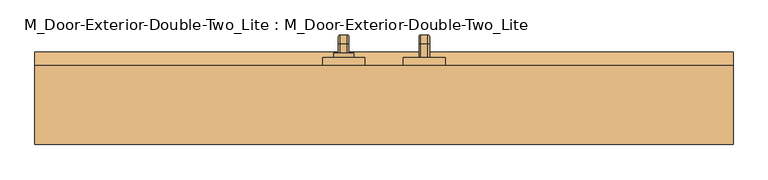
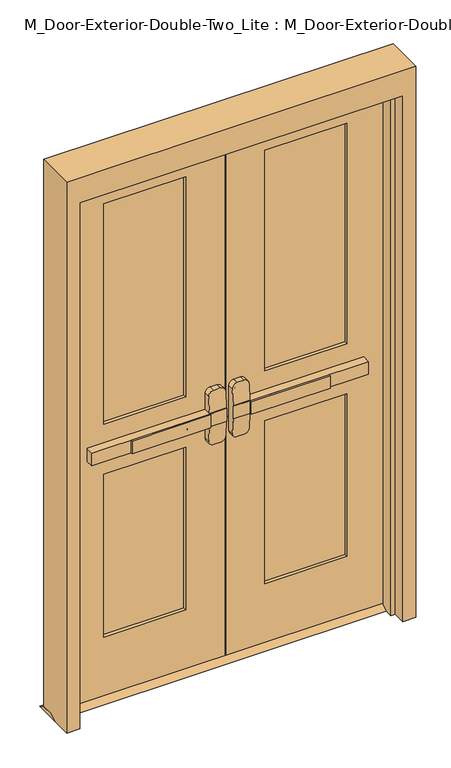
"""IFC4 building model written with IfcOpenShell, lengths in millimetres: door geometry, M_Door-Exterior-Double-Two_Lite : M_Door-Exterior-Double-Two_Lite."""

from ifc_helpers import new_model, si_unit, point, frame, frame_2d, origin, place, context, project, spatial, polyline, circle_curve, ellipse_curve, trimmed, segment, composite_curve, outline, extrude, faceted_brep, source, transform, mapped, element, save
from ifc_brep_helpers import plane_surface, cylinder_surface, revolved_surface, advanced_brep


def m_door_exterior_double_two_lite_m_door_exterior_double_two_f203ad21(model_context):
    return source(origin(), model_context, "Body", "SolidModel", [
        extrude(outline(polyline([(-373.6, 12.55), (-373.6, 18.9), (-76.2, 18.9), (-76.2, 12.55), (-373.6, 12.55)])), frame((0.0, 0.0, 974.6), z_axis=(0.0, 0.0, 1.0), x_axis=(1.0, 0.0, 0.0)), (0.0, 0.0, 1.0), 50.8),
        advanced_brep(
        [(-12.7, 18.9, 1025.4), (-76.2, 18.9, 1025.4), (-522.3, 18.9, 1025.4), (-522.3, 18.9, 974.6), (-76.2, 18.9, 974.6), (-12.7, 18.9, 974.6), (-522.3, 50.65, 1025.4), (-76.2, 50.65, 1025.4), (-76.2, 50.65, 1088.9), (-57.15, 50.65, 1107.95), (-31.75, 50.65, 1107.95), (-12.7, 50.65, 1088.9), (-12.7, 50.65, 911.1), (-31.75, 50.65, 892.05), (-57.15, 50.65, 892.05), (-76.2, 50.65, 911.1), (-76.2, 50.65, 974.6), (-522.3, 50.65, 974.6), (-12.7, 22.0752467, 1025.4), (-76.2, 22.0752467, 1025.4), (-12.7, 22.0752467, 974.6), (-12.7, 27.0854269, 911.1), (-12.7, 27.0854269, 1088.9), (-76.2, 22.0752467, 974.6), (-76.2, 27.0854269, 1088.9), (-76.2, 27.0854269, 911.1), (-57.15, 28.588481, 1107.95), (-31.75, 28.588481, 1107.95), (-31.75, 28.588481, 892.05), (-57.15, 28.588481, 892.05)],
        [
            (0, 1),
            (1, 2),
            (2, 3),
            (3, 4),
            (4, 5),
            (5, 0),
            (6, 7),
            (7, 8),
            (8, 9, circle_curve(frame((-57.15, 50.65, 1088.9), z_axis=(0.0, 1.0, 0.0), x_axis=(-1.0, 0.0, 0.0)), 19.05)),
            (9, 10),
            (10, 11, circle_curve(frame((-31.75, 50.65, 1088.9), z_axis=(0.0, 1.0, 0.0), x_axis=(-1.0, 0.0, 0.0)), 19.05)),
            (11, 12),
            (12, 13, circle_curve(frame((-31.75, 50.65, 911.1), z_axis=(0.0, 1.0, 0.0), x_axis=(-1.0, 0.0, 0.0)), 19.05)),
            (13, 14),
            (14, 15, circle_curve(frame((-57.15, 50.65, 911.1), z_axis=(0.0, 1.0, 0.0), x_axis=(-1.0, 0.0, 0.0)), 19.05)),
            (15, 16),
            (16, 17),
            (17, 6),
            (0, 18),
            (18, 19),
            (19, 7),
            (6, 2),
            (5, 20),
            (20, 21),
            (21, 12),
            (11, 22),
            (22, 18),
            (16, 23),
            (23, 20),
            (3, 17),
            (19, 24),
            (24, 8),
            (15, 25),
            (25, 23),
            (9, 26),
            (26, 27),
            (27, 10),
            (13, 28),
            (28, 29),
            (29, 14),
            (29, 25, ellipse_curve(frame((-57.15, 27.0854269, 911.1), z_axis=(0.0, 0.9969018152893365, 0.07865602756830282), x_axis=(0.0, -0.07865602756830208, 0.9969018152893365)), 19.1092038, 19.05)),
            (24, 26, ellipse_curve(frame((-57.15, 27.0854269, 1088.9), z_axis=(0.0, 0.9969018152893376, -0.07865602756828934), x_axis=(0.0, -0.078656027568288, -0.9969018152893377)), 19.1092038, 19.05)),
            (27, 22, ellipse_curve(frame((-31.75, 27.0854269, 1088.9), z_axis=(0.0, 0.9969018152893376, -0.07865602756828934), x_axis=(0.0, -0.078656027568288, -0.9969018152893377)), 19.1092038, 19.05)),
            (21, 28, ellipse_curve(frame((-31.75, 27.0854269, 911.1), z_axis=(0.0, 0.9969018152893365, 0.07865602756830282), x_axis=(0.0, -0.07865602756830208, 0.9969018152893365)), 19.1092038, 19.05)),
        ],
        [
            plane_surface(frame((-12.7, 18.9, 1025.4), z_axis=(0.0, -1.0, 0.0), x_axis=(1.0, 0.0, 0.0))),
            plane_surface(frame((-12.7, 50.65, 1025.4), z_axis=(0.0, 1.0, 0.0), x_axis=(-1.0, 0.0, 0.0))),
            plane_surface(frame((-522.3, 18.9, 1025.4), z_axis=(0.0, 0.0, 1.0), x_axis=(0.0, 1.0, 0.0))),
            plane_surface(frame((-12.7, 18.9, 1025.4), z_axis=(1.0, 0.0, 0.0), x_axis=(0.0, 1.0, 0.0))),
            plane_surface(frame((-12.7, 18.9, 974.6), z_axis=(0.0, 0.0, -1.0), x_axis=(0.0, 1.0, 0.0))),
            plane_surface(frame((-522.3, 18.9, 974.6), z_axis=(-1.0, 0.0, 0.0), x_axis=(0.0, 1.0, 0.0))),
            plane_surface(frame((-76.2, 22.0752467, 911.1), z_axis=(-1.0, 0.0, 0.0), x_axis=(0.0, 1.0, 0.0))),
            plane_surface(frame((-57.15, 22.0752467, 1107.95), z_axis=(0.0, 0.0, 1.0), x_axis=(0.0, 1.0, 0.0))),
            plane_surface(frame((-31.75, 22.0752467, 892.05), z_axis=(0.0, 0.0, -1.0), x_axis=(0.0, 1.0, 0.0))),
            cylinder_surface(frame((-57.15, 50.65, 911.1), z_axis=(0.0, -1.0, 0.0), x_axis=(-1.0, 0.0, 0.0)), 19.05),
            cylinder_surface(frame((-57.15, 50.65, 1088.9), z_axis=(0.0, -1.0, 0.0), x_axis=(-1.0, 0.0, 0.0)), 19.05),
            cylinder_surface(frame((-31.75, 50.65, 1088.9), z_axis=(0.0, -1.0, 0.0), x_axis=(-1.0, 0.0, 0.0)), 19.05),
            cylinder_surface(frame((-31.75, 50.65, 911.1), z_axis=(0.0, -1.0, 0.0), x_axis=(-1.0, 0.0, 0.0)), 19.05),
            plane_surface(frame((-76.2, 22.0752467, 1025.4), z_axis=(0.0, -0.9969018152893376, 0.07865602756828934), x_axis=(1.0, 0.0, 0.0))),
            plane_surface(frame((-76.2, 28.588481, 892.05), z_axis=(0.0, -0.9969018152893365, -0.07865602756830282), x_axis=(1.0, 0.0, 0.0))),
        ],
        [
            (0, [[1, 2, 3, 4, 5, 6]]),
            (1, [[7, 8, 9, 10, 11, 12, 13, 14, 15, 16, 17, 18]]),
            (2, [[-2, -1, 19, 20, 21, -7, 22]]),
            (3, [[23, 24, 25, -12, 26, 27, -19, -6]]),
            (4, [[-17, 28, 29, -23, -5, -4, 30]]),
            (5, [[-22, -18, -30, -3]]),
            (6, [[-21, 31, 32, -8]]),
            (6, [[33, 34, -28, -16]]),
            (7, [[35, 36, 37, -10]]),
            (8, [[38, 39, 40, -14]]),
            (9, [[-40, 41, -33, -15]]),
            (10, [[-32, 42, -35, -9]]),
            (11, [[-37, 43, -26, -11]]),
            (12, [[-25, 44, -38, -13]]),
            (13, [[-27, -43, -36, -42, -31, -20]]),
            (14, [[-29, -34, -41, -39, -44, -24]]),
        ],
    ),
        extrude(outline(polyline([(95.65, 15.0), (121.05, 0.0), (25.25, 0.0), (50.65, 15.0), (95.65, 15.0)])), frame((-659.6, 0.0, 0.0), z_axis=(1.0, 0.0, 0.0), x_axis=(0.0, 1.0, 0.0)), (0.0, 0.0, 1.0), 1319.2),
        extrude(outline(polyline([(373.6, 12.55), (76.2, 12.55), (76.2, 18.9), (373.6, 18.9), (373.6, 12.55)])), frame((0.0, 0.0, 974.6), z_axis=(0.0, 0.0, 1.0), x_axis=(1.0, 0.0, 0.0)), (0.0, 0.0, 1.0), 50.8),
        advanced_brep(
        [(12.7, 18.9, 1025.4), (12.7, 18.9, 974.6), (76.2, 18.9, 974.6), (522.3, 18.9, 974.6), (522.3, 18.9, 1025.4), (76.2, 18.9, 1025.4), (522.3, 50.65, 1025.4), (522.3, 50.65, 974.6), (76.2, 50.65, 974.6), (76.2, 50.65, 911.1), (57.15, 50.65, 892.05), (31.75, 50.65, 892.05), (12.7, 50.65, 911.1), (12.7, 50.65, 1088.9), (31.75, 50.65, 1107.95), (57.15, 50.65, 1107.95), (76.2, 50.65, 1088.9), (76.2, 50.65, 1025.4), (76.2, 22.0752467, 1025.4), (12.7, 22.0752467, 1025.4), (12.7, 27.0854269, 1088.9), (12.7, 27.0854269, 911.1), (12.7, 22.0752467, 974.6), (76.2, 22.0752467, 974.6), (76.2, 27.0854269, 911.1), (76.2, 27.0854269, 1088.9), (31.75, 28.588481, 1107.95), (57.15, 28.588481, 1107.95), (57.15, 28.588481, 892.05), (31.75, 28.588481, 892.05)],
        [
            (0, 1),
            (1, 2),
            (2, 3),
            (3, 4),
            (4, 5),
            (5, 0),
            (6, 7),
            (7, 8),
            (8, 9),
            (9, 10, circle_curve(frame((57.15, 50.65, 911.1), z_axis=(0.0, 1.0, 0.0), x_axis=(1.0, 0.0, 0.0)), 19.05)),
            (10, 11),
            (11, 12, circle_curve(frame((31.75, 50.65, 911.1), z_axis=(0.0, 1.0, 0.0), x_axis=(1.0, 0.0, 0.0)), 19.05)),
            (12, 13),
            (13, 14, circle_curve(frame((31.75, 50.65, 1088.9), z_axis=(0.0, 1.0, 0.0), x_axis=(1.0, 0.0, 0.0)), 19.05)),
            (14, 15),
            (15, 16, circle_curve(frame((57.15, 50.65, 1088.9), z_axis=(0.0, 1.0, 0.0), x_axis=(1.0, 0.0, 0.0)), 19.05)),
            (16, 17),
            (17, 6),
            (4, 6),
            (17, 18),
            (18, 19),
            (19, 0),
            (19, 20),
            (20, 13),
            (12, 21),
            (21, 22),
            (22, 1),
            (7, 3),
            (22, 23),
            (23, 8),
            (23, 24),
            (24, 9),
            (16, 25),
            (25, 18),
            (14, 26),
            (26, 27),
            (27, 15),
            (10, 28),
            (28, 29),
            (29, 11),
            (24, 28, ellipse_curve(frame((57.15, 27.0854269, 911.1), z_axis=(0.0, 0.9969018152893365, 0.07865602756830282), x_axis=(0.0, -0.07865602756830208, 0.9969018152893365)), 19.1092038, 19.05)),
            (27, 25, ellipse_curve(frame((57.15, 27.0854269, 1088.9), z_axis=(0.0, 0.9969018152893376, -0.07865602756828934), x_axis=(0.0, -0.078656027568288, -0.9969018152893377)), 19.1092038, 19.05)),
            (20, 26, ellipse_curve(frame((31.75, 27.0854269, 1088.9), z_axis=(0.0, 0.9969018152893376, -0.07865602756828934), x_axis=(0.0, -0.078656027568288, -0.9969018152893377)), 19.1092038, 19.05)),
            (29, 21, ellipse_curve(frame((31.75, 27.0854269, 911.1), z_axis=(0.0, 0.9969018152893365, 0.07865602756830282), x_axis=(0.0, -0.07865602756830208, 0.9969018152893365)), 19.1092038, 19.05)),
        ],
        [
            plane_surface(frame((12.7, 18.9, 1025.4), z_axis=(0.0, -1.0, 0.0), x_axis=(-1.0, 0.0, 0.0))),
            plane_surface(frame((12.7, 50.65, 1025.4), z_axis=(0.0, 1.0, 0.0), x_axis=(1.0, 0.0, 0.0))),
            plane_surface(frame((522.3, 18.9, 1025.4), z_axis=(0.0, 0.0, 1.0), x_axis=(0.0, 1.0, 0.0))),
            plane_surface(frame((12.7, 18.9, 1025.4), z_axis=(-1.0, 0.0, 0.0), x_axis=(0.0, 1.0, 0.0))),
            plane_surface(frame((12.7, 18.9, 974.6), z_axis=(0.0, 0.0, -1.0), x_axis=(0.0, 1.0, 0.0))),
            plane_surface(frame((522.3, 18.9, 974.6), z_axis=(1.0, 0.0, 0.0), x_axis=(0.0, 1.0, 0.0))),
            plane_surface(frame((76.2, 22.0752467, 911.1), z_axis=(1.0, 0.0, 0.0), x_axis=(0.0, 1.0, 0.0))),
            plane_surface(frame((57.15, 22.0752467, 1107.95), z_axis=(0.0, 0.0, 1.0), x_axis=(0.0, 1.0, 0.0))),
            plane_surface(frame((31.75, 22.0752467, 892.05), z_axis=(0.0, 0.0, -1.0), x_axis=(0.0, 1.0, 0.0))),
            cylinder_surface(frame((57.15, 50.65, 911.1), z_axis=(0.0, -1.0, 0.0), x_axis=(1.0, 0.0, 0.0)), 19.05),
            cylinder_surface(frame((57.15, 50.65, 1088.9), z_axis=(0.0, -1.0, 0.0), x_axis=(1.0, 0.0, 0.0)), 19.05),
            cylinder_surface(frame((31.75, 50.65, 1088.9), z_axis=(0.0, -1.0, 0.0), x_axis=(1.0, 0.0, 0.0)), 19.05),
            cylinder_surface(frame((31.75, 50.65, 911.1), z_axis=(0.0, -1.0, 0.0), x_axis=(1.0, 0.0, 0.0)), 19.05),
            plane_surface(frame((76.2, 22.0752467, 1025.4), z_axis=(0.0, -0.9969018152893376, 0.07865602756828934), x_axis=(-1.0, 0.0, 0.0))),
            plane_surface(frame((76.2, 28.588481, 892.05), z_axis=(0.0, -0.9969018152893365, -0.07865602756830282), x_axis=(-1.0, 0.0, 0.0))),
        ],
        [
            (0, [[1, 2, 3, 4, 5, 6]]),
            (1, [[7, 8, 9, 10, 11, 12, 13, 14, 15, 16, 17, 18]]),
            (2, [[19, -18, 20, 21, 22, -6, -5]]),
            (3, [[-1, -22, 23, 24, -13, 25, 26, 27]]),
            (4, [[28, -3, -2, -27, 29, 30, -8]]),
            (5, [[-4, -28, -7, -19]]),
            (6, [[-9, -30, 31, 32]]),
            (6, [[-17, 33, 34, -20]]),
            (7, [[-15, 35, 36, 37]]),
            (8, [[-11, 38, 39, 40]]),
            (9, [[-10, -32, 41, -38]]),
            (10, [[-16, -37, 42, -33]]),
            (11, [[-14, -24, 43, -35]]),
            (12, [[-12, -40, 44, -25]]),
            (13, [[-21, -34, -42, -36, -43, -23]]),
            (14, [[-26, -44, -39, -41, -31, -29]]),
        ],
    ),
        advanced_brep(
        [(66.2, 110.65, 1001.190625), (66.2, 110.65, 998.809375), (69.771875, 110.65, 995.2375), (82.6284594, 110.65, 995.2375), (86.2, 110.65, 998.8090406), (86.2, 110.65, 1001.190625), (82.628125, 110.65, 1004.7625), (69.771875, 110.65, 1004.7625), (66.2, 110.65, 874.609375), (69.771875, 110.65, 871.0375), (82.628125, 110.65, 871.0375), (86.2, 110.65, 874.609375), (86.2, 110.65, 876.9909594), (82.6284594, 110.65, 880.5625), (69.771875, 110.65, 880.5625), (66.2, 110.65, 876.990625), (66.2, 136.05, 1001.190625), (66.2, 149.940625, 987.3), (66.2, 149.940625, 888.5), (66.2, 136.05, 874.609375), (66.2, 136.05, 876.990625), (66.2, 147.559375, 888.5), (66.2, 147.559375, 987.3), (66.2, 136.05, 998.809375), (69.771875, 136.05, 995.2375), (82.6284594, 136.05, 995.2375), (86.2, 136.05, 998.8090406), (86.2, 147.5590406, 987.3), (86.2, 147.5590406, 888.5), (86.2, 136.05, 876.9909594), (86.2, 136.05, 874.609375), (86.2, 149.940625, 888.5), (86.2, 149.940625, 987.3), (86.2, 136.05, 1001.190625), (82.628125, 136.05, 1004.7625), (69.771875, 136.05, 1004.7625), (69.771875, 143.9875, 987.3), (82.6284594, 143.9875, 987.3), (82.628125, 153.5125, 987.3), (69.771875, 153.5125, 987.3), (69.771875, 143.9875, 888.5), (82.6284594, 143.9875, 888.5), (82.628125, 153.5125, 888.5), (69.771875, 153.5125, 888.5), (69.771875, 136.05, 880.5625), (82.6284594, 136.05, 880.5625), (82.628125, 136.05, 871.0375), (69.771875, 136.05, 871.0375)],
        [
            (0, 1),
            (1, 2, circle_curve(frame((69.771875, 110.65, 998.809375), z_axis=(0.0, -1.0, 0.0), x_axis=(0.0, 0.0, 1.0)), 3.571875)),
            (2, 3),
            (3, 4, circle_curve(frame((82.6284594, 110.65, 998.8090406), z_axis=(0.0, -1.0, 0.0), x_axis=(0.0, 0.0, 1.0)), 3.5715406)),
            (4, 5),
            (5, 6, circle_curve(frame((82.628125, 110.65, 1001.190625), z_axis=(0.0, -1.0, 0.0), x_axis=(0.0, 0.0, 1.0)), 3.571875)),
            (6, 7),
            (7, 0, circle_curve(frame((69.771875, 110.65, 1001.190625), z_axis=(0.0, -1.0, 0.0), x_axis=(0.0, 0.0, 1.0)), 3.571875)),
            (8, 9, circle_curve(frame((69.771875, 110.65, 874.609375), z_axis=(0.0, -1.0, 0.0), x_axis=(0.0, 0.0, -1.0)), 3.571875)),
            (9, 10),
            (10, 11, circle_curve(frame((82.628125, 110.65, 874.609375), z_axis=(0.0, -1.0, 0.0), x_axis=(0.0, 0.0, -1.0)), 3.571875)),
            (11, 12),
            (12, 13, circle_curve(frame((82.6284594, 110.65, 876.9909594), z_axis=(0.0, -1.0, 0.0), x_axis=(0.0, 0.0, -1.0)), 3.5715406)),
            (13, 14),
            (14, 15, circle_curve(frame((69.771875, 110.65, 876.990625), z_axis=(0.0, -1.0, 0.0), x_axis=(0.0, 0.0, -1.0)), 3.571875)),
            (15, 8),
            (0, 16),
            (16, 17, circle_curve(frame((66.2, 136.05, 987.3), z_axis=(-1.0, 0.0, 0.0), x_axis=(0.0, 0.0, 1.0)), 13.890625)),
            (17, 18),
            (18, 19, circle_curve(frame((66.2, 136.05, 888.5), z_axis=(-1.0, 0.0, 0.0), x_axis=(0.0, 1.0, 0.0)), 13.890625)),
            (19, 8),
            (15, 20),
            (20, 21, circle_curve(frame((66.2, 136.05, 888.5), z_axis=(1.0, 0.0, 0.0), x_axis=(0.0, 1.0, 0.0)), 11.509375)),
            (21, 22),
            (22, 23, circle_curve(frame((66.2, 136.05, 987.3), z_axis=(1.0, 0.0, 0.0), x_axis=(0.0, 0.0, 1.0)), 11.509375)),
            (23, 1),
            (23, 24, circle_curve(frame((69.771875, 136.05, 998.809375), z_axis=(0.0, -1.0, 0.0), x_axis=(0.0, 0.0, 1.0)), 3.571875)),
            (24, 2),
            (24, 25),
            (25, 3),
            (25, 26, circle_curve(frame((82.6284594, 136.05, 998.8090406), z_axis=(0.0, -1.0, 0.0), x_axis=(0.0, 0.0, 1.0)), 3.5715406)),
            (26, 4),
            (26, 27, circle_curve(frame((86.2, 136.05, 987.3), z_axis=(-1.0, 0.0, 0.0), x_axis=(0.0, 0.0, 1.0)), 11.5090406)),
            (27, 28),
            (28, 29, circle_curve(frame((86.2, 136.05, 888.5), z_axis=(-1.0, 0.0, 0.0), x_axis=(0.0, 1.0, 0.0)), 11.5090406)),
            (29, 12),
            (11, 30),
            (30, 31, circle_curve(frame((86.2, 136.05, 888.5), z_axis=(1.0, 0.0, 0.0), x_axis=(0.0, 1.0, 0.0)), 13.890625)),
            (31, 32),
            (32, 33, circle_curve(frame((86.2, 136.05, 987.3), z_axis=(1.0, 0.0, 0.0), x_axis=(0.0, 0.0, 1.0)), 13.890625)),
            (33, 5),
            (33, 34, circle_curve(frame((82.628125, 136.05, 1001.190625), z_axis=(0.0, -1.0, 0.0), x_axis=(0.0, 0.0, 1.0)), 3.571875)),
            (34, 6),
            (34, 35),
            (35, 7),
            (35, 16, circle_curve(frame((69.771875, 136.05, 1001.190625), z_axis=(0.0, -1.0, 0.0), x_axis=(0.0, 0.0, 1.0)), 3.571875)),
            (36, 24, circle_curve(frame((69.771875, 136.05, 987.3), z_axis=(1.0, 0.0, 0.0), x_axis=(0.0, 0.0, 1.0)), 7.9375)),
            (22, 36, circle_curve(frame((69.771875, 147.559375, 987.3), z_axis=(0.0, 0.0, 1.0), x_axis=(0.0, 1.0, 0.0)), 3.571875)),
            (37, 25, circle_curve(frame((82.6284594, 136.05, 987.3), z_axis=(1.0, 0.0, 0.0), x_axis=(0.0, 0.0, 1.0)), 7.9375)),
            (36, 37),
            (37, 27, circle_curve(frame((82.6284594, 147.5590406, 987.3), z_axis=(0.0, 0.0, 1.0), x_axis=(0.0, 1.0, 0.0)), 3.5715406)),
            (38, 34, circle_curve(frame((82.628125, 136.05, 987.3), z_axis=(1.0, 0.0, 0.0), x_axis=(0.0, 0.0, 1.0)), 17.4625)),
            (32, 38, circle_curve(frame((82.628125, 149.940625, 987.3), z_axis=(0.0, 0.0, 1.0), x_axis=(0.0, 1.0, 0.0)), 3.571875)),
            (39, 35, circle_curve(frame((69.771875, 136.05, 987.3), z_axis=(1.0, 0.0, 0.0), x_axis=(0.0, 0.0, 1.0)), 17.4625)),
            (38, 39),
            (39, 17, circle_curve(frame((69.771875, 149.940625, 987.3), z_axis=(0.0, 0.0, 1.0), x_axis=(0.0, 1.0, 0.0)), 3.571875)),
            (21, 40, circle_curve(frame((69.771875, 147.559375, 888.5), z_axis=(0.0, 0.0, 1.0), x_axis=(0.0, 1.0, 0.0)), 3.571875)),
            (40, 36),
            (40, 41),
            (41, 37),
            (41, 28, circle_curve(frame((82.6284594, 147.5590406, 888.5), z_axis=(0.0, 0.0, 1.0), x_axis=(0.0, 1.0, 0.0)), 3.5715406)),
            (31, 42, circle_curve(frame((82.628125, 149.940625, 888.5), z_axis=(0.0, 0.0, 1.0), x_axis=(0.0, 1.0, 0.0)), 3.571875)),
            (42, 38),
            (42, 43),
            (43, 39),
            (43, 18, circle_curve(frame((69.771875, 149.940625, 888.5), z_axis=(0.0, 0.0, 1.0), x_axis=(0.0, 1.0, 0.0)), 3.571875)),
            (44, 40, circle_curve(frame((69.771875, 136.05, 888.5), z_axis=(1.0, 0.0, 0.0), x_axis=(0.0, 1.0, 0.0)), 7.9375)),
            (20, 44, circle_curve(frame((69.771875, 136.05, 876.990625), z_axis=(0.0, 1.0, 0.0), x_axis=(0.0, 0.0, -1.0)), 3.571875)),
            (45, 41, circle_curve(frame((82.6284594, 136.05, 888.5), z_axis=(1.0, 0.0, 0.0), x_axis=(0.0, 1.0, 0.0)), 7.9375)),
            (44, 45),
            (45, 29, circle_curve(frame((82.6284594, 136.05, 876.9909594), z_axis=(0.0, 1.0, 0.0), x_axis=(0.0, 0.0, -1.0)), 3.5715406)),
            (46, 42, circle_curve(frame((82.628125, 136.05, 888.5), z_axis=(1.0, 0.0, 0.0), x_axis=(0.0, 1.0, 0.0)), 17.4625)),
            (30, 46, circle_curve(frame((82.628125, 136.05, 874.609375), z_axis=(0.0, 1.0, 0.0), x_axis=(0.0, 0.0, -1.0)), 3.571875)),
            (47, 43, circle_curve(frame((69.771875, 136.05, 888.5), z_axis=(1.0, 0.0, 0.0), x_axis=(0.0, 1.0, 0.0)), 17.4625)),
            (46, 47),
            (47, 19, circle_curve(frame((69.771875, 136.05, 874.609375), z_axis=(0.0, 1.0, 0.0), x_axis=(0.0, 0.0, -1.0)), 3.571875)),
            (14, 44),
            (13, 45),
            (10, 46),
            (9, 47),
        ],
        [
            plane_surface(frame((76.2, 110.65, 1000.0), z_axis=(0.0, -1.0, 0.0), x_axis=(1.0, 0.0, 0.0))),
            plane_surface(frame((76.2, 110.65, 875.8), z_axis=(0.0, -1.0, 0.0), x_axis=(1.0, 0.0, 0.0))),
            plane_surface(frame((66.2, 110.65, 1001.190625), z_axis=(-1.0, 0.0, 0.0), x_axis=(0.0, 1.0, 0.0))),
            cylinder_surface(frame((69.771875, 110.65, 998.809375), z_axis=(0.0, -1.0, 0.0), x_axis=(0.0, 0.0, 1.0)), 3.571875),
            plane_surface(frame((69.771875, 110.65, 995.2375), z_axis=(0.0, 0.0, -1.0), x_axis=(0.0, 1.0, 0.0))),
            cylinder_surface(frame((82.6284594, 110.65, 998.8090406), z_axis=(0.0, -1.0, 0.0), x_axis=(0.0, 0.0, 1.0)), 3.5715406),
            plane_surface(frame((86.2, 110.65, 998.8090406), z_axis=(1.0, 0.0, 0.0), x_axis=(0.0, 1.0, 0.0))),
            cylinder_surface(frame((82.628125, 110.65, 1001.190625), z_axis=(0.0, -1.0, 0.0), x_axis=(0.0, 0.0, 1.0)), 3.571875),
            plane_surface(frame((82.628125, 110.65, 1004.7625), z_axis=(0.0, 0.0, 1.0), x_axis=(0.0, 1.0, 0.0))),
            cylinder_surface(frame((69.771875, 110.65, 1001.190625), z_axis=(0.0, -1.0, 0.0), x_axis=(0.0, 0.0, 1.0)), 3.571875),
            revolved_surface(trimmed(ellipse_curve(frame((69.771875, 136.05, 998.809375), z_axis=(0.0, -1.0, 0.0), x_axis=(0.0, 0.0, 1.0)), 3.571875, 3.571875), [point((66.2, 136.05, 998.809375))], [point((69.771875, 136.05, 995.2375))], True, "CARTESIAN"), (76.2, 136.05, 987.3), (-1.0, 0.0, 0.0)),
            revolved_surface(polyline([(69.771875, 136.05, 995.2375), (82.6284594, 136.05, 995.2375)]), (76.2, 136.05, 987.3), (-1.0, 0.0, 0.0)),
            revolved_surface(trimmed(ellipse_curve(frame((82.6284594, 136.05, 998.8090406), z_axis=(0.0, -1.0, 0.0), x_axis=(0.0, 0.0, 1.0)), 3.5715406, 3.5715406), [point((82.6284594, 136.05, 995.2375))], [point((86.2, 136.05, 998.8090406))], True, "CARTESIAN"), (76.2, 136.05, 987.3), (-1.0, 0.0, 0.0)),
            revolved_surface(trimmed(ellipse_curve(frame((82.628125, 136.05, 1001.190625), z_axis=(0.0, -1.0, 0.0), x_axis=(0.0, 0.0, 1.0)), 3.571875, 3.571875), [point((86.2, 136.05, 1001.190625))], [point((82.628125, 136.05, 1004.7625))], True, "CARTESIAN"), (76.2, 136.05, 987.3), (-1.0, 0.0, 0.0)),
            cylinder_surface(frame((76.2, 136.05, 987.3), z_axis=(-1.0, 0.0, 0.0), x_axis=(0.0, 0.0, 1.0)), 17.4625),
            revolved_surface(trimmed(ellipse_curve(frame((69.771875, 136.05, 1001.190625), z_axis=(0.0, -1.0, 0.0), x_axis=(0.0, 0.0, 1.0)), 3.571875, 3.571875), [point((69.771875, 136.05, 1004.7625))], [point((66.2, 136.05, 1001.190625))], True, "CARTESIAN"), (76.2, 136.05, 987.3), (-1.0, 0.0, 0.0)),
            cylinder_surface(frame((69.771875, 147.559375, 987.3), z_axis=(0.0, 0.0, 1.0), x_axis=(0.0, 1.0, 0.0)), 3.571875),
            plane_surface(frame((69.771875, 143.9875, 987.3), z_axis=(0.0, -1.0, 0.0), x_axis=(0.0, 0.0, -1.0))),
            cylinder_surface(frame((82.6284594, 147.5590406, 987.3), z_axis=(0.0, 0.0, 1.0), x_axis=(0.0, 1.0, 0.0)), 3.5715406),
            cylinder_surface(frame((82.628125, 149.940625, 987.3), z_axis=(0.0, 0.0, 1.0), x_axis=(0.0, 1.0, 0.0)), 3.571875),
            plane_surface(frame((82.628125, 153.5125, 987.3), z_axis=(0.0, 1.0, 0.0), x_axis=(0.0, 0.0, -1.0))),
            cylinder_surface(frame((69.771875, 149.940625, 987.3), z_axis=(0.0, 0.0, 1.0), x_axis=(0.0, 1.0, 0.0)), 3.571875),
            revolved_surface(trimmed(ellipse_curve(frame((69.771875, 147.559375, 888.5), z_axis=(0.0, 0.0, 1.0), x_axis=(0.0, 1.0, 0.0)), 3.571875, 3.571875), [point((66.2, 147.559375, 888.5))], [point((69.771875, 143.9875, 888.5))], True, "CARTESIAN"), (76.2, 136.05, 888.5), (-1.0, 0.0, 0.0)),
            revolved_surface(polyline([(69.771875, 143.9875, 888.5), (82.6284594, 143.9875, 888.5)]), (76.2, 136.05, 888.5), (-1.0, 0.0, 0.0)),
            revolved_surface(trimmed(ellipse_curve(frame((82.6284594, 147.5590406, 888.5), z_axis=(0.0, 0.0, 1.0), x_axis=(0.0, 1.0, 0.0)), 3.5715406, 3.5715406), [point((82.6284594, 143.9875, 888.5))], [point((86.2, 147.5590406, 888.5))], True, "CARTESIAN"), (76.2, 136.05, 888.5), (-1.0, 0.0, 0.0)),
            revolved_surface(trimmed(ellipse_curve(frame((82.628125, 149.940625, 888.5), z_axis=(0.0, 0.0, 1.0), x_axis=(0.0, 1.0, 0.0)), 3.571875, 3.571875), [point((86.2, 149.940625, 888.5))], [point((82.628125, 153.5125, 888.5))], True, "CARTESIAN"), (76.2, 136.05, 888.5), (-1.0, 0.0, 0.0)),
            cylinder_surface(frame((76.2, 136.05, 888.5), z_axis=(-1.0, 0.0, 0.0), x_axis=(0.0, 1.0, 0.0)), 17.4625),
            revolved_surface(trimmed(ellipse_curve(frame((69.771875, 149.940625, 888.5), z_axis=(0.0, 0.0, 1.0), x_axis=(0.0, 1.0, 0.0)), 3.571875, 3.571875), [point((69.771875, 153.5125, 888.5))], [point((66.2, 149.940625, 888.5))], True, "CARTESIAN"), (76.2, 136.05, 888.5), (-1.0, 0.0, 0.0)),
            cylinder_surface(frame((69.771875, 136.05, 876.990625), z_axis=(0.0, 1.0, 0.0), x_axis=(0.0, 0.0, -1.0)), 3.571875),
            plane_surface(frame((69.771875, 136.05, 880.5625), z_axis=(0.0, 0.0, 1.0), x_axis=(0.0, -1.0, 0.0))),
            cylinder_surface(frame((82.6284594, 136.05, 876.9909594), z_axis=(0.0, 1.0, 0.0), x_axis=(0.0, 0.0, -1.0)), 3.5715406),
            cylinder_surface(frame((82.628125, 136.05, 874.609375), z_axis=(0.0, 1.0, 0.0), x_axis=(0.0, 0.0, -1.0)), 3.571875),
            plane_surface(frame((82.628125, 136.05, 871.0375), z_axis=(0.0, 0.0, -1.0), x_axis=(0.0, -1.0, 0.0))),
            cylinder_surface(frame((69.771875, 136.05, 874.609375), z_axis=(0.0, 1.0, 0.0), x_axis=(0.0, 0.0, -1.0)), 3.571875),
        ],
        [
            (0, [[1, 2, 3, 4, 5, 6, 7, 8]]),
            (1, [[9, 10, 11, 12, 13, 14, 15, 16]]),
            (2, [[-1, 17, 18, 19, 20, 21, -16, 22, 23, 24, 25, 26]]),
            (3, [[-2, -26, 27, 28]]),
            (4, [[-3, -28, 29, 30]]),
            (5, [[-4, -30, 31, 32]]),
            (6, [[-5, -32, 33, 34, 35, 36, -12, 37, 38, 39, 40, 41]]),
            (7, [[-6, -41, 42, 43]]),
            (8, [[-7, -43, 44, 45]]),
            (9, [[-8, -45, 46, -17]]),
            (10, [[47, -27, -25, 48]]),
            (11, [[49, -29, -47, 50]]),
            (12, [[-33, -31, -49, 51]]),
            (13, [[52, -42, -40, 53]]),
            (14, [[54, -44, -52, 55]]),
            (15, [[-18, -46, -54, 56]]),
            (16, [[-48, -24, 57, 58]]),
            (17, [[-50, -58, 59, 60]]),
            (18, [[-51, -60, 61, -34]]),
            (19, [[-53, -39, 62, 63]]),
            (20, [[-55, -63, 64, 65]]),
            (21, [[-56, -65, 66, -19]]),
            (22, [[67, -57, -23, 68]]),
            (23, [[69, -59, -67, 70]]),
            (24, [[-35, -61, -69, 71]]),
            (25, [[72, -62, -38, 73]]),
            (26, [[74, -64, -72, 75]]),
            (27, [[-20, -66, -74, 76]]),
            (28, [[-68, -22, -15, 77]]),
            (29, [[-70, -77, -14, 78]]),
            (30, [[-71, -78, -13, -36]]),
            (31, [[-73, -37, -11, 79]]),
            (32, [[-75, -79, -10, 80]]),
            (33, [[-76, -80, -9, -21]]),
        ],
    ),
        extrude(outline(composite_curve([segment(trimmed(circle_curve(frame_2d((1094.2338574, 76.2)), 90.1286291), [point((1175.0, 116.2))], [point((1175.0, 36.2))], False, "CARTESIAN"), True, "CONTINUOUS"), segment(polyline([(1175.0, 36.2), (825.0, 36.2)]), True, "CONTINUOUS"), segment(trimmed(circle_curve(frame_2d((905.7661426, 76.2)), 90.1286291), [point((825.0, 36.2))], [point((825.0, 116.2))], False, "CARTESIAN"), True, "CONTINUOUS"), segment(polyline([(825.0, 116.2), (1175.0, 116.2)]), True, "CONTINUOUS")], self_intersect=False)), frame((0.0, 95.65, 0.0), z_axis=(0.0, 1.0, 0.0), x_axis=(0.0, 0.0, 1.0)), (0.0, 0.0, 1.0), 15.0),
        advanced_brep(
        [(-86.2, 110.65, 1001.190625), (-86.2, 110.65, 998.809375), (-82.628125, 110.65, 995.2375), (-69.7715406, 110.65, 995.2375), (-66.2, 110.65, 998.8090406), (-66.2, 110.65, 1001.190625), (-69.771875, 110.65, 1004.7625), (-82.628125, 110.65, 1004.7625), (-86.2, 110.65, 874.609375), (-82.628125, 110.65, 871.0375), (-69.771875, 110.65, 871.0375), (-66.2, 110.65, 874.609375), (-66.2, 110.65, 876.9909594), (-69.7715406, 110.65, 880.5625), (-82.628125, 110.65, 880.5625), (-86.2, 110.65, 876.990625), (-86.2, 136.05, 1001.190625), (-86.2, 149.940625, 987.3), (-86.2, 149.940625, 888.5), (-86.2, 136.05, 874.609375), (-86.2, 136.05, 876.990625), (-86.2, 147.559375, 888.5), (-86.2, 147.559375, 987.3), (-86.2, 136.05, 998.809375), (-82.628125, 136.05, 995.2375), (-69.7715406, 136.05, 995.2375), (-66.2, 136.05, 998.8090406), (-66.2, 147.5590406, 987.3), (-66.2, 147.5590406, 888.5), (-66.2, 136.05, 876.9909594), (-66.2, 136.05, 874.609375), (-66.2, 149.940625, 888.5), (-66.2, 149.940625, 987.3), (-66.2, 136.05, 1001.190625), (-69.771875, 136.05, 1004.7625), (-82.628125, 136.05, 1004.7625), (-82.628125, 143.9875, 987.3), (-69.7715406, 143.9875, 987.3), (-69.771875, 153.5125, 987.3), (-82.628125, 153.5125, 987.3), (-82.628125, 143.9875, 888.5), (-69.7715406, 143.9875, 888.5), (-69.771875, 153.5125, 888.5), (-82.628125, 153.5125, 888.5), (-82.628125, 136.05, 880.5625), (-69.7715406, 136.05, 880.5625), (-69.771875, 136.05, 871.0375), (-82.628125, 136.05, 871.0375)],
        [
            (0, 1),
            (1, 2, circle_curve(frame((-82.628125, 110.65, 998.809375), z_axis=(0.0, -1.0, 0.0), x_axis=(0.0, 0.0, 1.0)), 3.571875)),
            (2, 3),
            (3, 4, circle_curve(frame((-69.7715406, 110.65, 998.8090406), z_axis=(0.0, -1.0, 0.0), x_axis=(0.0, 0.0, 1.0)), 3.5715406)),
            (4, 5),
            (5, 6, circle_curve(frame((-69.771875, 110.65, 1001.190625), z_axis=(0.0, -1.0, 0.0), x_axis=(0.0, 0.0, 1.0)), 3.571875)),
            (6, 7),
            (7, 0, circle_curve(frame((-82.628125, 110.65, 1001.190625), z_axis=(0.0, -1.0, 0.0), x_axis=(0.0, 0.0, 1.0)), 3.571875)),
            (8, 9, circle_curve(frame((-82.628125, 110.65, 874.609375), z_axis=(0.0, -1.0, 0.0), x_axis=(0.0, 0.0, -1.0)), 3.571875)),
            (9, 10),
            (10, 11, circle_curve(frame((-69.771875, 110.65, 874.609375), z_axis=(0.0, -1.0, 0.0), x_axis=(0.0, 0.0, -1.0)), 3.571875)),
            (11, 12),
            (12, 13, circle_curve(frame((-69.7715406, 110.65, 876.9909594), z_axis=(0.0, -1.0, 0.0), x_axis=(0.0, 0.0, -1.0)), 3.5715406)),
            (13, 14),
            (14, 15, circle_curve(frame((-82.628125, 110.65, 876.990625), z_axis=(0.0, -1.0, 0.0), x_axis=(0.0, 0.0, -1.0)), 3.571875)),
            (15, 8),
            (0, 16),
            (16, 17, circle_curve(frame((-86.2, 136.05, 987.3), z_axis=(-1.0, 0.0, 0.0), x_axis=(0.0, 0.0, 1.0)), 13.890625)),
            (17, 18),
            (18, 19, circle_curve(frame((-86.2, 136.05, 888.5), z_axis=(-1.0, 0.0, 0.0), x_axis=(0.0, 1.0, 0.0)), 13.890625)),
            (19, 8),
            (15, 20),
            (20, 21, circle_curve(frame((-86.2, 136.05, 888.5), z_axis=(1.0, 0.0, 0.0), x_axis=(0.0, 1.0, 0.0)), 11.509375)),
            (21, 22),
            (22, 23, circle_curve(frame((-86.2, 136.05, 987.3), z_axis=(1.0, 0.0, 0.0), x_axis=(0.0, 0.0, 1.0)), 11.509375)),
            (23, 1),
            (23, 24, circle_curve(frame((-82.628125, 136.05, 998.809375), z_axis=(0.0, -1.0, 0.0), x_axis=(0.0, 0.0, 1.0)), 3.571875)),
            (24, 2),
            (24, 25),
            (25, 3),
            (25, 26, circle_curve(frame((-69.7715406, 136.05, 998.8090406), z_axis=(0.0, -1.0, 0.0), x_axis=(0.0, 0.0, 1.0)), 3.5715406)),
            (26, 4),
            (26, 27, circle_curve(frame((-66.2, 136.05, 987.3), z_axis=(-1.0, 0.0, 0.0), x_axis=(0.0, 0.0, 1.0)), 11.5090406)),
            (27, 28),
            (28, 29, circle_curve(frame((-66.2, 136.05, 888.5), z_axis=(-1.0, 0.0, 0.0), x_axis=(0.0, 1.0, 0.0)), 11.5090406)),
            (29, 12),
            (11, 30),
            (30, 31, circle_curve(frame((-66.2, 136.05, 888.5), z_axis=(1.0, 0.0, 0.0), x_axis=(0.0, 1.0, 0.0)), 13.890625)),
            (31, 32),
            (32, 33, circle_curve(frame((-66.2, 136.05, 987.3), z_axis=(1.0, 0.0, 0.0), x_axis=(0.0, 0.0, 1.0)), 13.890625)),
            (33, 5),
            (33, 34, circle_curve(frame((-69.771875, 136.05, 1001.190625), z_axis=(0.0, -1.0, 0.0), x_axis=(0.0, 0.0, 1.0)), 3.571875)),
            (34, 6),
            (34, 35),
            (35, 7),
            (35, 16, circle_curve(frame((-82.628125, 136.05, 1001.190625), z_axis=(0.0, -1.0, 0.0), x_axis=(0.0, 0.0, 1.0)), 3.571875)),
            (36, 24, circle_curve(frame((-82.628125, 136.05, 987.3), z_axis=(1.0, 0.0, 0.0), x_axis=(0.0, 0.0, 1.0)), 7.9375)),
            (22, 36, circle_curve(frame((-82.628125, 147.559375, 987.3), z_axis=(0.0, 0.0, 1.0), x_axis=(0.0, 1.0, 0.0)), 3.571875)),
            (37, 25, circle_curve(frame((-69.7715406, 136.05, 987.3), z_axis=(1.0, 0.0, 0.0), x_axis=(0.0, 0.0, 1.0)), 7.9375)),
            (36, 37),
            (37, 27, circle_curve(frame((-69.7715406, 147.5590406, 987.3), z_axis=(0.0, 0.0, 1.0), x_axis=(0.0, 1.0, 0.0)), 3.5715406)),
            (38, 34, circle_curve(frame((-69.771875, 136.05, 987.3), z_axis=(1.0, 0.0, 0.0), x_axis=(0.0, 0.0, 1.0)), 17.4625)),
            (32, 38, circle_curve(frame((-69.771875, 149.940625, 987.3), z_axis=(0.0, 0.0, 1.0), x_axis=(0.0, 1.0, 0.0)), 3.571875)),
            (39, 35, circle_curve(frame((-82.628125, 136.05, 987.3), z_axis=(1.0, 0.0, 0.0), x_axis=(0.0, 0.0, 1.0)), 17.4625)),
            (38, 39),
            (39, 17, circle_curve(frame((-82.628125, 149.940625, 987.3), z_axis=(0.0, 0.0, 1.0), x_axis=(0.0, 1.0, 0.0)), 3.571875)),
            (21, 40, circle_curve(frame((-82.628125, 147.559375, 888.5), z_axis=(0.0, 0.0, 1.0), x_axis=(0.0, 1.0, 0.0)), 3.571875)),
            (40, 36),
            (40, 41),
            (41, 37),
            (41, 28, circle_curve(frame((-69.7715406, 147.5590406, 888.5), z_axis=(0.0, 0.0, 1.0), x_axis=(0.0, 1.0, 0.0)), 3.5715406)),
            (31, 42, circle_curve(frame((-69.771875, 149.940625, 888.5), z_axis=(0.0, 0.0, 1.0), x_axis=(0.0, 1.0, 0.0)), 3.571875)),
            (42, 38),
            (42, 43),
            (43, 39),
            (43, 18, circle_curve(frame((-82.628125, 149.940625, 888.5), z_axis=(0.0, 0.0, 1.0), x_axis=(0.0, 1.0, 0.0)), 3.571875)),
            (44, 40, circle_curve(frame((-82.628125, 136.05, 888.5), z_axis=(1.0, 0.0, 0.0), x_axis=(0.0, 1.0, 0.0)), 7.9375)),
            (20, 44, circle_curve(frame((-82.628125, 136.05, 876.990625), z_axis=(0.0, 1.0, 0.0), x_axis=(0.0, 0.0, -1.0)), 3.571875)),
            (45, 41, circle_curve(frame((-69.7715406, 136.05, 888.5), z_axis=(1.0, 0.0, 0.0), x_axis=(0.0, 1.0, 0.0)), 7.9375)),
            (44, 45),
            (45, 29, circle_curve(frame((-69.7715406, 136.05, 876.9909594), z_axis=(0.0, 1.0, 0.0), x_axis=(0.0, 0.0, -1.0)), 3.5715406)),
            (46, 42, circle_curve(frame((-69.771875, 136.05, 888.5), z_axis=(1.0, 0.0, 0.0), x_axis=(0.0, 1.0, 0.0)), 17.4625)),
            (30, 46, circle_curve(frame((-69.771875, 136.05, 874.609375), z_axis=(0.0, 1.0, 0.0), x_axis=(0.0, 0.0, -1.0)), 3.571875)),
            (47, 43, circle_curve(frame((-82.628125, 136.05, 888.5), z_axis=(1.0, 0.0, 0.0), x_axis=(0.0, 1.0, 0.0)), 17.4625)),
            (46, 47),
            (47, 19, circle_curve(frame((-82.628125, 136.05, 874.609375), z_axis=(0.0, 1.0, 0.0), x_axis=(0.0, 0.0, -1.0)), 3.571875)),
            (14, 44),
            (13, 45),
            (10, 46),
            (9, 47),
        ],
        [
            plane_surface(frame((-76.2, 110.65, 1000.0), z_axis=(0.0, -1.0, 0.0), x_axis=(1.0, 0.0, 0.0))),
            plane_surface(frame((-76.2, 110.65, 875.8), z_axis=(0.0, -1.0, 0.0), x_axis=(1.0, 0.0, 0.0))),
            plane_surface(frame((-86.2, 110.65, 1001.190625), z_axis=(-1.0, 0.0, 0.0), x_axis=(0.0, 1.0, 0.0))),
            cylinder_surface(frame((-82.628125, 110.65, 998.809375), z_axis=(0.0, -1.0, 0.0), x_axis=(0.0, 0.0, 1.0)), 3.571875),
            plane_surface(frame((-82.628125, 110.65, 995.2375), z_axis=(0.0, 0.0, -1.0), x_axis=(0.0, 1.0, 0.0))),
            cylinder_surface(frame((-69.7715406, 110.65, 998.8090406), z_axis=(0.0, -1.0, 0.0), x_axis=(0.0, 0.0, 1.0)), 3.5715406),
            plane_surface(frame((-66.2, 110.65, 998.8090406), z_axis=(1.0, 0.0, 0.0), x_axis=(0.0, 1.0, 0.0))),
            cylinder_surface(frame((-69.771875, 110.65, 1001.190625), z_axis=(0.0, -1.0, 0.0), x_axis=(0.0, 0.0, 1.0)), 3.571875),
            plane_surface(frame((-69.771875, 110.65, 1004.7625), z_axis=(0.0, 0.0, 1.0), x_axis=(0.0, 1.0, 0.0))),
            cylinder_surface(frame((-82.628125, 110.65, 1001.190625), z_axis=(0.0, -1.0, 0.0), x_axis=(0.0, 0.0, 1.0)), 3.571875),
            revolved_surface(trimmed(ellipse_curve(frame((-82.628125, 136.05, 998.809375), z_axis=(0.0, -1.0, 0.0), x_axis=(0.0, 0.0, 1.0)), 3.571875, 3.571875), [point((-86.2, 136.05, 998.809375))], [point((-82.628125, 136.05, 995.2375))], True, "CARTESIAN"), (-76.2, 136.05, 987.3), (-1.0, 0.0, 0.0)),
            revolved_surface(polyline([(-82.628125, 136.05, 995.2375), (-69.7715406, 136.05, 995.2375)]), (-76.2, 136.05, 987.3), (-1.0, 0.0, 0.0)),
            revolved_surface(trimmed(ellipse_curve(frame((-69.7715406, 136.05, 998.8090406), z_axis=(0.0, -1.0, 0.0), x_axis=(0.0, 0.0, 1.0)), 3.5715406, 3.5715406), [point((-69.7715406, 136.05, 995.2375))], [point((-66.2, 136.05, 998.8090406))], True, "CARTESIAN"), (-76.2, 136.05, 987.3), (-1.0, 0.0, 0.0)),
            revolved_surface(trimmed(ellipse_curve(frame((-69.771875, 136.05, 1001.190625), z_axis=(0.0, -1.0, 0.0), x_axis=(0.0, 0.0, 1.0)), 3.571875, 3.571875), [point((-66.2, 136.05, 1001.190625))], [point((-69.771875, 136.05, 1004.7625))], True, "CARTESIAN"), (-76.2, 136.05, 987.3), (-1.0, 0.0, 0.0)),
            cylinder_surface(frame((-76.2, 136.05, 987.3), z_axis=(-1.0, 0.0, 0.0), x_axis=(0.0, 0.0, 1.0)), 17.4625),
            revolved_surface(trimmed(ellipse_curve(frame((-82.628125, 136.05, 1001.190625), z_axis=(0.0, -1.0, 0.0), x_axis=(0.0, 0.0, 1.0)), 3.571875, 3.571875), [point((-82.628125, 136.05, 1004.7625))], [point((-86.2, 136.05, 1001.190625))], True, "CARTESIAN"), (-76.2, 136.05, 987.3), (-1.0, 0.0, 0.0)),
            cylinder_surface(frame((-82.628125, 147.559375, 987.3), z_axis=(0.0, 0.0, 1.0), x_axis=(0.0, 1.0, 0.0)), 3.571875),
            plane_surface(frame((-82.628125, 143.9875, 987.3), z_axis=(0.0, -1.0, 0.0), x_axis=(0.0, 0.0, -1.0))),
            cylinder_surface(frame((-69.7715406, 147.5590406, 987.3), z_axis=(0.0, 0.0, 1.0), x_axis=(0.0, 1.0, 0.0)), 3.5715406),
            cylinder_surface(frame((-69.771875, 149.940625, 987.3), z_axis=(0.0, 0.0, 1.0), x_axis=(0.0, 1.0, 0.0)), 3.571875),
            plane_surface(frame((-69.771875, 153.5125, 987.3), z_axis=(0.0, 1.0, 0.0), x_axis=(0.0, 0.0, -1.0))),
            cylinder_surface(frame((-82.628125, 149.940625, 987.3), z_axis=(0.0, 0.0, 1.0), x_axis=(0.0, 1.0, 0.0)), 3.571875),
            revolved_surface(trimmed(ellipse_curve(frame((-82.628125, 147.559375, 888.5), z_axis=(0.0, 0.0, 1.0), x_axis=(0.0, 1.0, 0.0)), 3.571875, 3.571875), [point((-86.2, 147.559375, 888.5))], [point((-82.628125, 143.9875, 888.5))], True, "CARTESIAN"), (-76.2, 136.05, 888.5), (-1.0, 0.0, 0.0)),
            revolved_surface(polyline([(-82.628125, 143.9875, 888.5), (-69.7715406, 143.9875, 888.5)]), (-76.2, 136.05, 888.5), (-1.0, 0.0, 0.0)),
            revolved_surface(trimmed(ellipse_curve(frame((-69.7715406, 147.5590406, 888.5), z_axis=(0.0, 0.0, 1.0), x_axis=(0.0, 1.0, 0.0)), 3.5715406, 3.5715406), [point((-69.7715406, 143.9875, 888.5))], [point((-66.2, 147.5590406, 888.5))], True, "CARTESIAN"), (-76.2, 136.05, 888.5), (-1.0, 0.0, 0.0)),
            revolved_surface(trimmed(ellipse_curve(frame((-69.771875, 149.940625, 888.5), z_axis=(0.0, 0.0, 1.0), x_axis=(0.0, 1.0, 0.0)), 3.571875, 3.571875), [point((-66.2, 149.940625, 888.5))], [point((-69.771875, 153.5125, 888.5))], True, "CARTESIAN"), (-76.2, 136.05, 888.5), (-1.0, 0.0, 0.0)),
            cylinder_surface(frame((-76.2, 136.05, 888.5), z_axis=(-1.0, 0.0, 0.0), x_axis=(0.0, 1.0, 0.0)), 17.4625),
            revolved_surface(trimmed(ellipse_curve(frame((-82.628125, 149.940625, 888.5), z_axis=(0.0, 0.0, 1.0), x_axis=(0.0, 1.0, 0.0)), 3.571875, 3.571875), [point((-82.628125, 153.5125, 888.5))], [point((-86.2, 149.940625, 888.5))], True, "CARTESIAN"), (-76.2, 136.05, 888.5), (-1.0, 0.0, 0.0)),
            cylinder_surface(frame((-82.628125, 136.05, 876.990625), z_axis=(0.0, 1.0, 0.0), x_axis=(0.0, 0.0, -1.0)), 3.571875),
            plane_surface(frame((-82.628125, 136.05, 880.5625), z_axis=(0.0, 0.0, 1.0), x_axis=(0.0, -1.0, 0.0))),
            cylinder_surface(frame((-69.7715406, 136.05, 876.9909594), z_axis=(0.0, 1.0, 0.0), x_axis=(0.0, 0.0, -1.0)), 3.5715406),
            cylinder_surface(frame((-69.771875, 136.05, 874.609375), z_axis=(0.0, 1.0, 0.0), x_axis=(0.0, 0.0, -1.0)), 3.571875),
            plane_surface(frame((-69.771875, 136.05, 871.0375), z_axis=(0.0, 0.0, -1.0), x_axis=(0.0, -1.0, 0.0))),
            cylinder_surface(frame((-82.628125, 136.05, 874.609375), z_axis=(0.0, 1.0, 0.0), x_axis=(0.0, 0.0, -1.0)), 3.571875),
        ],
        [
            (0, [[1, 2, 3, 4, 5, 6, 7, 8]]),
            (1, [[9, 10, 11, 12, 13, 14, 15, 16]]),
            (2, [[-1, 17, 18, 19, 20, 21, -16, 22, 23, 24, 25, 26]]),
            (3, [[-2, -26, 27, 28]]),
            (4, [[-3, -28, 29, 30]]),
            (5, [[-4, -30, 31, 32]]),
            (6, [[-5, -32, 33, 34, 35, 36, -12, 37, 38, 39, 40, 41]]),
            (7, [[-6, -41, 42, 43]]),
            (8, [[-7, -43, 44, 45]]),
            (9, [[-8, -45, 46, -17]]),
            (10, [[47, -27, -25, 48]]),
            (11, [[49, -29, -47, 50]]),
            (12, [[-33, -31, -49, 51]]),
            (13, [[52, -42, -40, 53]]),
            (14, [[54, -44, -52, 55]]),
            (15, [[-18, -46, -54, 56]]),
            (16, [[-48, -24, 57, 58]]),
            (17, [[-50, -58, 59, 60]]),
            (18, [[-51, -60, 61, -34]]),
            (19, [[-53, -39, 62, 63]]),
            (20, [[-55, -63, 64, 65]]),
            (21, [[-56, -65, 66, -19]]),
            (22, [[67, -57, -23, 68]]),
            (23, [[69, -59, -67, 70]]),
            (24, [[-35, -61, -69, 71]]),
            (25, [[72, -62, -38, 73]]),
            (26, [[74, -64, -72, 75]]),
            (27, [[-20, -66, -74, 76]]),
            (28, [[-68, -22, -15, 77]]),
            (29, [[-70, -77, -14, 78]]),
            (30, [[-71, -78, -13, -36]]),
            (31, [[-73, -37, -11, 79]]),
            (32, [[-75, -79, -10, 80]]),
            (33, [[-76, -80, -9, -21]]),
        ],
    ),
        extrude(outline(composite_curve([segment(trimmed(circle_curve(frame_2d((1098.8, -76.2)), 19.0), [point((1098.8, -95.2))], [point((1098.8, -57.2))], False, "CARTESIAN"), True, "CONTINUOUS"), segment(trimmed(circle_curve(frame_2d((1098.8, -76.2)), 19.0), [point((1098.8, -57.2))], [point((1098.8, -95.2))], False, "CARTESIAN"), True, "CONTINUOUS")], self_intersect=False)), frame((0.0, 110.65, 0.0), z_axis=(0.0, 1.0, 0.0), x_axis=(0.0, 0.0, 1.0)), (0.0, 0.0, 1.0), 8.73125),
        extrude(outline(composite_curve([segment(trimmed(circle_curve(frame_2d((1094.2338574, -76.2)), 90.1286291), [point((1175.0, -36.2))], [point((1175.0, -116.2))], False, "CARTESIAN"), True, "CONTINUOUS"), segment(polyline([(1175.0, -116.2), (825.0, -116.2)]), True, "CONTINUOUS"), segment(trimmed(circle_curve(frame_2d((905.7661426, -76.2)), 90.1286291), [point((825.0, -116.2))], [point((825.0, -36.2))], False, "CARTESIAN"), True, "CONTINUOUS"), segment(polyline([(825.0, -36.2), (1175.0, -36.2)]), True, "CONTINUOUS")], self_intersect=False)), frame((0.0, 95.65, 0.0), z_axis=(0.0, 1.0, 0.0), x_axis=(0.0, 0.0, 1.0)), (0.0, 0.0, 1.0), 15.0),
        extrude(outline(polyline([(2100.0, 1.5875), (15.0, 1.5875), (15.0, 609.6), (2100.0, 609.6), (2100.0, 1.5875)]), holes=[polyline([(1980.0, 150.0), (1980.0, 459.6), (1100.0, 459.6), (1100.0, 150.0), (1980.0, 150.0)]), polyline([(900.0, 150.0), (900.0, 459.6), (250.0, 459.6), (250.0, 150.0), (900.0, 150.0)])]), frame((0.0, 50.65, 0.0), z_axis=(0.0, 1.0, 0.0), x_axis=(0.0, 0.0, 1.0)), (0.0, 0.0, 1.0), 45.0),
        extrude(outline(polyline([(15.0, -1.5875), (2100.0, -1.5875), (2100.0, -609.6), (15.0, -609.6), (15.0, -1.5875)]), holes=[polyline([(1980.0, -459.6), (1980.0, -150.0), (1100.0, -150.0), (1100.0, -459.6), (1980.0, -459.6)]), polyline([(900.0, -459.6), (900.0, -150.0), (250.0, -150.0), (250.0, -459.6), (900.0, -459.6)])]), frame((0.0, 50.65, 0.0), z_axis=(0.0, 1.0, 0.0), x_axis=(0.0, 0.0, 1.0)), (0.0, 0.0, 1.0), 45.0),
        faceted_brep([(609.6, 45.8875, 0.0), (609.6, 95.65, 0.0), (659.6, 95.65, 0.0), (659.6, -54.35, 0.0), (609.6, -54.35, 0.0), (609.6, -5.1375, 0.0), (593.725, -5.1375, 0.0), (593.725, 45.8875, 0.0), (609.6, 45.8875, 2100.0), (609.6, 95.65, 2100.0), (-609.6, 95.65, 2100.0), (-609.6, 95.65, 0.0), (-659.6, 95.65, 0.0), (-659.6, 95.65, 2200.0), (659.6, 95.65, 2200.0), (659.6, -54.35, 2200.0), (-659.6, -54.35, 2200.0), (-659.6, -54.35, 0.0), (-609.6, -54.35, 0.0), (-609.6, -54.35, 2100.0), (609.6, -54.35, 2100.0), (609.6, -5.1375, 2100.0), (-609.6, -5.1375, 2100.0), (-609.6, -5.1375, 0.0), (-593.725, -5.1375, 0.0), (-593.725, -5.1375, 2084.125), (593.725, -5.1375, 2084.125), (593.725, 45.8875, 2084.125), (-593.725, 45.8875, 2084.125), (-593.725, 45.8875, 0.0), (-609.6, 45.8875, 0.0), (-609.6, 45.8875, 2100.0)], [[[0, 1, 2, 3, 4, 5, 6, 7]], [[1, 0, 8, 9]], [[2, 1, 9, 10, 11, 12, 13, 14]], [[3, 2, 14, 15]], [[4, 3, 15, 16, 17, 18, 19, 20]], [[5, 4, 20, 21]], [[6, 5, 21, 22, 23, 24, 25, 26]], [[7, 6, 26, 27]], [[0, 7, 27, 28, 29, 30, 31, 8]], [[9, 8, 31, 10]], [[20, 19, 22, 21]], [[26, 25, 28, 27]], [[12, 11, 30, 29, 24, 23, 18, 17]], [[11, 10, 31, 30]], [[13, 12, 17, 16]], [[19, 18, 23, 22]], [[25, 24, 29, 28]], [[15, 14, 13, 16]]]),
        extrude(outline(polyline([(459.6, 63.15), (150.0, 63.15), (150.0, 83.15), (459.6, 83.15), (459.6, 63.15)])), frame((0.0, 0.0, 1100.0), z_axis=(0.0, 0.0, 1.0), x_axis=(1.0, 0.0, 0.0)), (0.0, 0.0, 1.0), 880.0),
        extrude(outline(polyline([(-150.0, 63.15), (-459.6, 63.15), (-459.6, 83.15), (-150.0, 83.15), (-150.0, 63.15)])), frame((0.0, 0.0, 1100.0), z_axis=(0.0, 0.0, 1.0), x_axis=(1.0, 0.0, 0.0)), (0.0, 0.0, 1.0), 880.0),
        extrude(outline(polyline([(-150.0, 63.15), (-459.6, 63.15), (-459.6, 83.15), (-150.0, 83.15), (-150.0, 63.15)])), frame((0.0, 0.0, 250.0), z_axis=(0.0, 0.0, 1.0), x_axis=(1.0, 0.0, 0.0)), (0.0, 0.0, 1.0), 650.0),
        extrude(outline(polyline([(459.6, 63.15), (150.0, 63.15), (150.0, 83.15), (459.6, 83.15), (459.6, 63.15)])), frame((0.0, 0.0, 250.0), z_axis=(0.0, 0.0, 1.0), x_axis=(1.0, 0.0, 0.0)), (0.0, 0.0, 1.0), 650.0),
    ])


if __name__ == "__main__":
    model = new_model("IFC4")
    model_context = context("Model", 3, world=origin())
    ifc_project = project(units=[si_unit("LENGTHUNIT", "METRE", prefix="MILLI")], contexts=[model_context])
    site = spatial("IfcSite", under=ifc_project)
    building = spatial("IfcBuilding", under=site)
    placement = place(None, origin())
    m_door_exterior_double_two_lite_m_door_exterior_double_two_shape = m_door_exterior_double_two_lite_m_door_exterior_double_two_f203ad21(model_context)
    element("IfcDoor", 1, ObjectType="M_Door-Exterior-Double-Two_Lite : M_Door-Exterior-Double-Two_Lite", at=placement, inside=building, context=model_context, shape_type="MappedRepresentation", body=[
        mapped(m_door_exterior_double_two_lite_m_door_exterior_double_two_shape, transform((0.0, 0.0, 0.0), x_axis=(1.0, 0.0, 0.0), y_axis=(0.0, 1.0, 0.0), z_axis=(0.0, 0.0, 1.0))),
    ])
    save(model, "model.ifc")

# Revit data of these elements
# Type "M_Door-Exterior-Double-Two_Lite : M_Door-Exterior-Double-Two_Lite"
#   Type Mark = "8"
#   Assembly Code = "B2030100"
#   Analytic Construction = "Metal frame, double glass door"
#   Top Rail = 0' - 4.72441"
#   Threshold Length [instance default] = 4' - 3.93701"
#   Threshold Offset [instance default] = 0' - 0.59055"
#   Thickness = 0' - 1.77165"
#   Thermal Resistance (R) = 1.3794 (h·ft²·°F)/BTU
#   Swing Angle [instance default] = 90.00°
#   Strike Height = 3' - 3.37008"
#   Stiles = 0' - 5.90551"
#   SinglePanelWidth = 2' - 0"
#   Rough Width [instance default] = 4' - 3.93701"
#   Rough Height [instance default] = 7' - 2.61417"
#   MFOpeningHeight [instance default] = 0' - 3.93701"
#   MFOpeningWidth [instance default] = 0' - 3.93701"
#   Lock Rail = 0' - 7.87402"
#   Inset Calculate [instance default] = 0' - 4.13386"
#   Masonry Inset [instance default] = 0' - 0.98425"
#   Height = 6' - 10.67717"
#   Width = 4' - 0"
#   Heat Transfer Coefficient (U) = 0.7250 BTU/(h·ft²·°F)
#   Glass Thickness = 0' - 0.7874"
#   Masonry Frame Depth = 0' - 5.90551"
#   Bottom Rail = 0' - 9.84252"
#   Threshold [instance default] = yes
#   Masonry Frame [instance default] = yes
#   Function = 1
#   Dry Wall Frame [instance default] = no
#   Threshold Material = Cherry
#   Panic Bar Material = Metal - Stainless Steel
#   Panel Material = Metal - Painted - Grey
#   Glass Stop Material = Metal - Painted - Grey
#   Frame Material = Metal - Painted - Grey
#   Exterior Pull Material = Metal - Stainless Steel
#   Visual Light Transmittance = 0
#   Solar Heat Gain Coefficient = 0
#   Wall Closure = (empty or 0)
# Element 1 (IfcDoor, "M_Door-Exterior-Double-Two_Lite : M_Door-Exterior-Double-Two_Lite")
#   Materials on its faces: "Metal - Painted - Grey", "Metal - Stainless Steel", "Glass", "Cherry"
# Materials
#   "Cherry": class "Wood", colour RGB 226 177 128, transparency 0, Description = "Prunus Serotina", Cost = 0
#   "Metal - Stainless Steel": class "Metal", colour RGB 247 247 247, transparency 0
#   "Metal - Painted - Grey": class "Paint", colour RGB 104 104 104, transparency 0, Cost = 0
#   "Glass": class "Glass", colour RGB 0 128 192, transparency 0.75, Description = "Soda Lime Glass", Cost = 0
